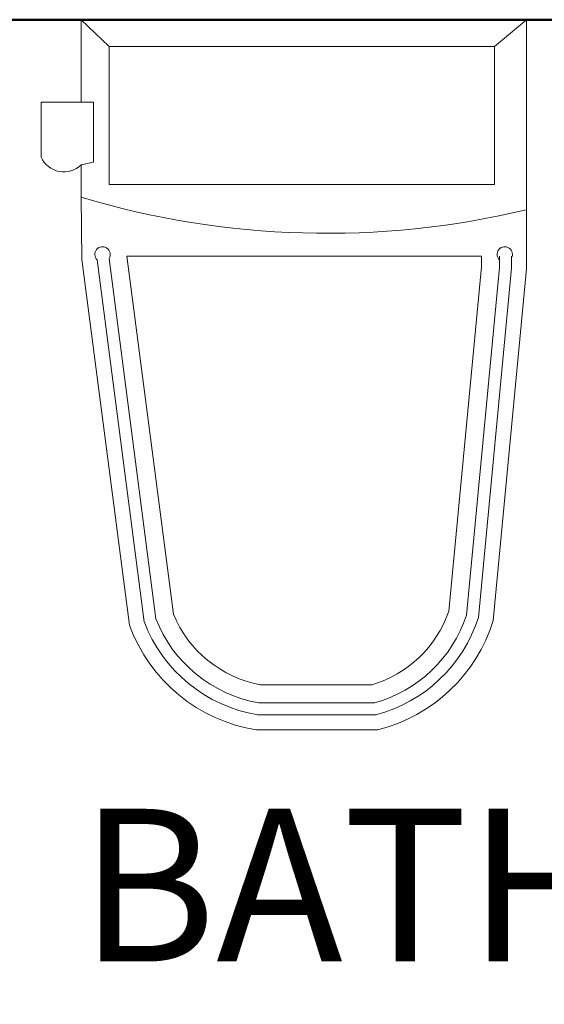
# Model space of a CAD drawing. Units: inches. Extents: x 64 to 1167, y 117 to 939.
# Tile 17 of 56: x 199 to 220, y 819 to 857. Entities that reach past the tile are written whole.
import ezdxf

# ---------------------------------------------------------------- set-up
doc = ezdxf.new("R2010")
doc.units = ezdxf.units.IN
doc.header["$MEASUREMENT"] = 0
for name, color, linetype, lineweight in [('A-ANNO-TEXT', 7, 'Continuous', 25), ('A-DOOR', 4, 'Continuous', 25), ('A-FLOR-FIXT', 8, 'Continuous', 18), ('A-WALL', 7, 'Continuous', 50)]:
    doc.layers.add(name, color=color, linetype=linetype, lineweight=lineweight)
doc.styles.get("Standard").update_dxf_attribs({"font": 'arial.ttf'})

# ---------------------------------------------------------------- blocks, each defined once
blk = doc.blocks.new('A$C68901CC0')
for p, q in [((10.955, 26.616), (12.347, 28.008)), ((12.347, 28.008), (37.402, 2.953)), ((36.01, 1.561), (10.955, 26.616)), ((0, 2.953), (0, 0)), ((1.969, 2.953), (0, 2.953)), ((1.969, 0), (1.969, 2.953)), ((37.402, 2.953), (36.01, 1.561)), ((37.402, 2.953), (37.402, 0)), ((39.37, 2.953), (37.402, 2.953)), ((39.37, 0), (39.37, 2.953)), ((0, 0), (1.969, 0)), ((37.402, 0), (39.37, 0))]:
    blk.add_line(p, q)
blk.add_arc((37.402, 2.953), 35.433, 135, 180)
blk = doc.blocks.new('A$C2B992F40')
for p, q in [((39.23, 615.24), (39.23, 696.15)), ((39.23, 696.15), (475.68, 696.15)), ((66.85, 669.73), (39.23, 696.15)), ((444.23, 669.73), (475.68, 696.15)), ((475.68, 696.15), (475.68, 509.8)), ((66.85, 534.62), (66.85, 669.73)), ((66.85, 669.73), (444.23, 669.73)), ((444.23, 669.73), (444.23, 534.62)), ((0, 561.3), (0, 615.24)), ((0, 615.24), (51.49, 615.24)), ((51.49, 615.24), (51.49, 556.39)), ((51.49, 556.39), (39.23, 553.94)), ((39.23, 522.06), (39.23, 553.94)), ((444.23, 534.62), (66.85, 534.62)), ((40.06, 461.24), (39.23, 522.06)), ((475.68, 509.8), (475.68, 451.92)), ((84.15, 464.39), (431.55, 464.39)), ((129.73, 113.43), (84.15, 464.39)), ((431.55, 464.39), (431.55, 454.01)), ((449.2, 464.39), (449.2, 453.17)), ((460.97, 464.39), (460.97, 452.62)), ((86.65, 102.5), (40.06, 461.24)), ((101.02, 106.05), (54.98, 460.61)), ((112.51, 108.95), (66.65, 462.12)), ((431.55, 454.01), (399.59, 116.19)), ((449.2, 453.17), (416.97, 112.48)), ((460.97, 452.62), (428.57, 110.08)), ((475.68, 451.92), (443.06, 107.16)), ((324.19, 44.13), (215, 44.13)), ((326.66, 26.48), (213.44, 26.48)), ((328.22, 14.71), (212.45, 14.71)), ((330.08, 0), (211.28, 0))]:
    blk.add_line(p, q)
for centre, radius, start, end in [((22.2, 571.41), 24.4, 204.49972, 314.26101), ((280.26, 1327.83), 841.04, 253.34642, 283.43557), ((60.2, 466.07), 7.56, 328.52932, 226.26991), ((454.43, 466.07), 7.56, 328.52932, 226.26991), ((291.54, 153.78), 114.41, 286.5809, 340.81554), ((235.93, 157), 132.44, 201.26818, 260.22173), ((235.93, 157), 114.79, 202.30203, 259.4948), ((291.54, 153.78), 132.06, 285.42576, 341.7737), ((291.54, 153.78), 143.83, 284.77755, 342.31156), ((291.54, 153.78), 158.54, 284.07165, 342.89742), ((235.93, 157), 158.92, 200.05507, 261.07522), ((235.93, 157), 144.21, 200.68762, 260.63012)]:
    blk.add_arc(centre, radius, start, end)

msp = doc.modelspace()

# ---------------------------------------------------------------- linework, layer by layer
at = {"layer": 'A-WALL'}
msp.add_line((297.107, 857.2), (183.107, 857.2), dxfattribs=at)

# ---------------------------------------------------------------- block references
at = {"layer": 'A-DOOR', "xscale": 0.837864491618382, "yscale": 0.837864491618382, "zscale": 0.837864491618382, "rotation": 270}
msp.add_blockref('A$C68901CC0', (179.107, 821.03), dxfattribs=at)
at = {"layer": 'A-FLOR-FIXT', "xscale": 0.0393700787401575, "yscale": 0.0393700787401575, "zscale": 0.0393700787401575}
msp.add_blockref('A$C2B992F40', (200.174, 829.792), dxfattribs=at)

# ---------------------------------------------------------------- texts
at = {"layer": 'A-ANNO-TEXT'}
msp.add_text('BATH ROOM', height=5.8926, dxfattribs=at).set_placement((201.648, 820.852))

doc.saveas('drawing.dxf')
